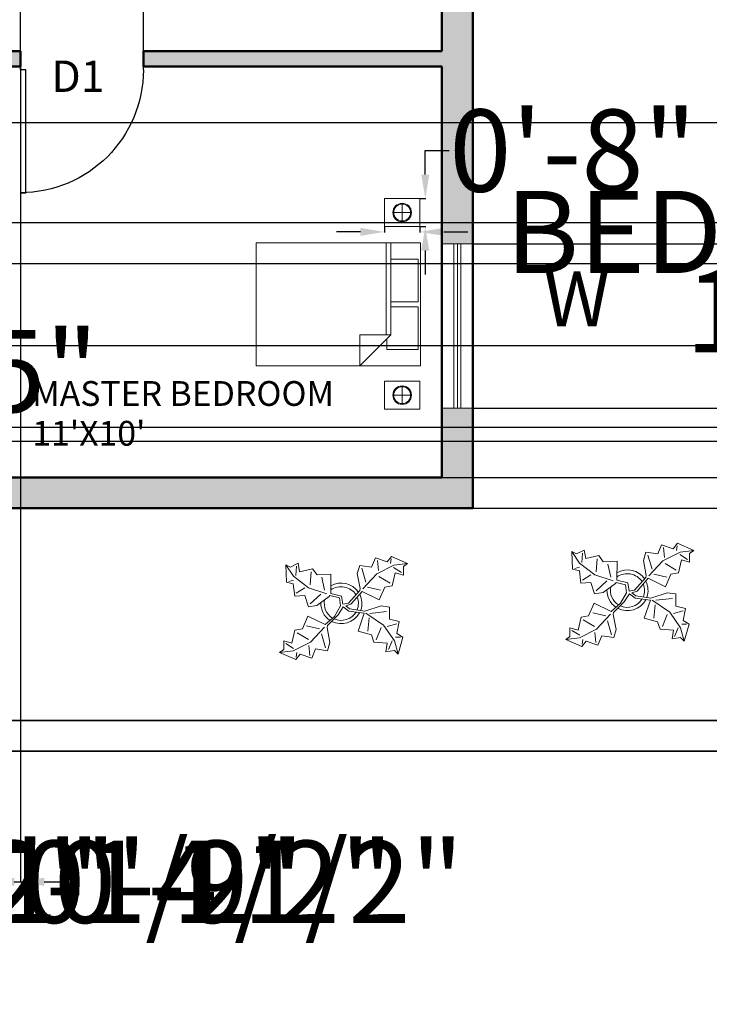
# Model space of a CAD drawing. Units: inches. Extents: x -166 to 1001, y 0 to 688.
# Tile 4 of 11: x 406 to 608, y 0 to 287. Entities that reach past the tile are written whole.
import ezdxf

# ---------------------------------------------------------------- set-up
doc = ezdxf.new("R2010")
doc.units = ezdxf.units.IN
doc.header["$MEASUREMENT"] = 0
for name, color, linetype, lineweight in [('A-ANNO-DIMS', 1, 'Continuous', 18), ('A-ANNO-TEXT', 2, 'Continuous', 25), ('A-AREA-IDEN', 2, 'Continuous', 25), ('A-DOOR', 6, 'Continuous', 25), ('A-GLAZ', 130, 'Continuous', 18), ('A-WALL-PATT', 5, 'Continuous', 13), ('C-SITE-WALL', 250, 'Continuous', 35), ('FURNITURE', 11, 'Continuous', 18), ('TREES', 80, 'Continuous', 13), ('WALLS', 250, 'Continuous', 50)]:
    doc.layers.add(name, color=color, linetype=linetype, lineweight=lineweight)
doc.styles.get("Standard").update_dxf_attribs({"font": 'arial.ttf'})
doc.dimstyles.get("Standard").update_dxf_attribs({"dimtxt": 24, "dimasz": 7, "dimexe": 0.18, "dimexo": 0.0625, "dimgap": 0.09, "dimtad": 0, "dimtih": 1, "dimtoh": 1, "dimdec": 0, "dimzin": 0, "dimdsep": 46, "dimlunit": 3, "dimtxsty": 'Standard', "dimcen": 0.09, "dimadec": 0, "dimazin": 0, "dimtfac": 1, "dimtdec": 0, "dimtofl": 0, "dimtmove": 0, "dimatfit": 3, "dimfxl": 1, "dimtolj": 1, "dimtzin": 0, "dimarcsym": 0})

# ---------------------------------------------------------------- blocks, each defined once
blk = doc.blocks.new('*U6')
for p, q in [((0, 0), (0, -6)), ((40, 0), (40, -6))]:
    blk.add_line(p, q)
blk.add_lwpolyline([(0, 0), (0, 40), (1.75, 40), (1.75, 0)], close=True)
blk.add_arc((0, 0), 40, 0, 90)
blk = doc.blocks.new('Bed - Queen')
for p, q in [((0, -80.00003), (0, 0)), ((0, 0), (59.99999, 0)), ((59.99999, 0), (59.99999, -80.00003)), ((7.99999, -1.2), (28.79998, -1.2)), ((7.99999, -14.4), (7.99999, -1.2)), ((28.79998, -1.2), (28.79998, -14.4)), ((31.19999, -1.2), (51.99999, -1.2)), ((31.19999, -14.4), (31.19999, -1.2)), ((51.99999, -1.2), (51.99999, -16.4)), ((0, -14.4), (44.8, -14.4)), ((44.8, -16.8), (0, -16.8)), ((59.99999, -29.6), (44.8, -14.4)), ((44.8, -14.4), (44.8, -29.6)), ((51.99999, -16.4), (46.79936, -16.4)), ((44.8, -29.6), (59.99999, -29.6)), ((59.99999, -80.00003), (0, -80.00003))]:
    blk.add_line(p, q)
blk = doc.blocks.new('Plant - Rubber or Philodendron')
for p, q in [((-14.8639, 10.7964), (-12.6195, 11.8975)), ((-12.6195, 11.8975), (-12.1909, 9.4345)), ((8.8871, 10.7908), (9.9809, 13.4933)), ((9.9809, 13.4933), (13.3837, 12.301)), ((10.5828, 12.6946), (10.8893, 9.7953)), ((13.3837, 12.301), (14.68, 13.9039)), ((14.5816, 13.2037), (14.3848, 11.8033)), ((14.68, 13.9039), (19.3848, 11.8146)), ((19.3848, 11.8146), (15.3859, 11.3055)), ((19.3848, 11.8146), (18.1868, 10.9119)), ((-16.2005, 11.4774), (-13.9899, 8.1064)), ((-16.2005, 11.4774), (-14.8639, 10.7964)), ((-16.0159, 6.3329), (-16.2005, 11.4774)), ((-13.3174, 8.325), (-13.0735, 11.0065)), ((-12.1909, 9.4345), (-8.3829, 10.3)), ((-8.8369, 9.409), (-9.0894, 5.6095)), ((-8.3829, 10.3), (-7.0549, 8.501)), ((-7.0549, 8.501), (-3.0284, 8.6941)), ((-3.0284, 8.6941), (-3.0709, 3.1041)), ((4.6914, 8.8812), (5.3859, 11.2828)), ((4.6914, 8.8812), (5.5014, 4.4831)), ((5.3859, 11.2828), (8.8871, 10.7908)), ((5.9878, 10.4842), (7.1971, 6.3869)), ((10.3916, 8.7942), (6.2847, 4.4028)), ((15.3859, 11.3055), (10.3916, 8.7942)), ((15.7909, 9.1065), (14.8995, 5.3044)), ((15.2875, 10.6053), (17.5907, 9.2105)), ((18.1925, 8.4119), (15.7909, 9.1065)), ((18.1868, 10.9119), (18.1925, 8.4119)), ((-14.0069, 5.8704), (-16.0159, 6.3329)), ((-15.3434, 6.5514), (-13.9984, 6.9884)), ((-13.5868, 2.2894), (-14.0069, 5.8704)), ((-13.9899, 8.1064), (-9.5434, 4.7185)), ((-4.8529, 4.012), (-5.7184, 7.82)), ((14.2977, 6.1031), (10.9934, 7.9956)), ((-13.1329, 3.1804), (-10.6614, 4.727)), ((-9.5434, 4.7185), (-4.1917, 2.9888)), ((-9.1318, 0.0195), (-5.9793, 2.9025)), ((-3.0709, 3.1041), (0.0797, 2.3163)), ((2.1141, 0.2298), (5.4346, 3.9146)), ((6.1032, 3.6844), (2.8262, -0.031)), ((5.4346, 3.9146), (5.5014, 4.4831)), ((11.1089, 1.1958), (6.1032, 3.6844)), ((7.7005, 4.8881), (11.5025, 3.9967)), ((12.7005, 4.8994), (11.1089, 1.1958)), ((14.8995, 5.3044), (12.7005, 4.8994)), ((-10.6784, 2.491), (-13.5868, 2.2894)), ((-9.5858, -0.8715), (-10.6784, 2.491)), ((-7.1228, -0.443), (-3.5248, 2.2131)), ((-3.5248, 2.2131), (-3.3011, 2.4355)), ((-3.3011, 2.4355), (-0.5306, 1.7947)), ((-0.5306, 1.7947), (-0.2255, -0.5527)), ((-0.5306, 1.7947), (-0.5306, 1.7947)), ((0.0797, 2.3163), (0.4866, -0.031)), ((0.4866, -0.031), (2.1141, 0.2298)), ((-7.1228, -0.443), (-9.5858, -0.8715)), ((-2.019, -3.6148), (-0.2255, -0.5527)), ((-0.9375, -3.1608), (0.5883, -0.8135)), ((0.5883, -0.8135), (2.2447, -2.0916)), ((2.8262, -0.031), (1.3003, -0.5527)), ((1.3003, -0.5527), (2.4193, -1.4655)), ((2.2447, -2.0916), (6.7108, -2.6626)), ((2.4193, -1.4655), (6.895, -2.1175)), ((4.943, -7.9659), (6.7108, -2.6626)), ((11.6605, -0.5413), (6.895, -2.1175)), ((12.3677, -6.1981), (7.219, -2.6772)), ((8.3544, -2.7453), (13.1973, -2.1704)), ((11.6605, -0.5413), (14.1354, -0.8948)), ((14.1354, -0.8948), (14.1354, -4.4304)), ((-11.3237, -7.2629), (-9.7321, -3.5593)), ((-9.7321, -3.5593), (-4.7264, -6.0479)), ((-2.019, -3.6148), (-4.7264, -6.0479)), ((-4.0579, -6.2781), (-0.9375, -3.1608)), ((8.125, -4.0768), (7.7715, -7.9659)), ((14.1354, -4.4304), (16.9638, -5.1375)), ((16.9638, -5.1375), (16.2567, -8.673)), ((-14.4141, -11.4699), (-13.5228, -7.6679)), ((-13.5228, -7.6679), (-11.3237, -7.2629)), ((-12.921, -8.4665), (-9.6166, -10.359)), ((-6.3237, -7.2516), (-10.1257, -6.3602)), ((-9.0148, -11.1577), (-4.9047, -6.8122)), ((-4.1246, -6.8466), (-4.0579, -6.2781)), ((-3.3146, -11.2447), (-4.1246, -6.8466)), ((8.8321, -9.0266), (4.943, -7.9659)), ((10.2463, -10.4408), (11.6605, -6.9053)), ((15.5496, -10.7943), (12.3677, -6.1981)), ((16.2567, -5.8446), (13.4283, -6.5517)), ((-16.8157, -10.7754), (-14.4141, -11.4699)), ((-16.8101, -13.2754), (-16.8157, -10.7754)), ((-14.0091, -13.669), (-9.0148, -11.1577)), ((-4.611, -12.8477), (-5.8203, -8.7504)), ((-3.3146, -11.2447), (-4.0092, -13.6463)), ((9.5392, -11.1479), (8.8321, -9.0266)), ((13.4283, -11.5015), (9.5392, -11.1479)), ((13.0748, -13.9763), (13.4283, -11.5015)), ((14.8425, -10.7943), (13.7819, -13.2692)), ((16.6103, -14.6834), (15.5496, -10.7943)), ((17.3174, -9.7337), (15.9032, -9.7337)), ((16.2567, -8.673), (18.0245, -9.7337)), ((18.0245, -9.7337), (16.6103, -14.6834)), ((-18.008, -14.1781), (-16.8101, -13.2754)), ((-18.008, -14.1781), (-14.0091, -13.669)), ((-13.3032, -16.2674), (-18.008, -14.1781)), ((-13.9107, -12.9688), (-16.2139, -11.574)), ((-13.2048, -15.5672), (-13.008, -14.1668)), ((-9.206, -15.0581), (-9.5126, -12.1588)), ((-7.5103, -13.1543), (-8.6042, -15.8568)), ((-4.0092, -13.6463), (-7.5103, -13.1543)), ((15.5496, -13.6228), (13.0748, -13.9763)), ((16.6103, -14.6834), (15.5496, -13.6228)), ((-12.0069, -14.6645), (-13.3032, -16.2674)), ((-8.6042, -15.8568), (-12.0069, -14.6645))]:
    blk.add_line(p, q)
for centre, radius, start, end in [((0, 0), 6.1275, 34.37569, 120.1028), ((-0.0601, -0.2075), 5.2461, 33.82192, 124.9414), ((0.0308, 0.1664), 6, 178.6147, 235.1169), ((0.0308, 0.1664), 5, 168.1647, 238.6725), ((-0.2664, 0.1682), 5.2775, 338.4094, 20.03007), ((-0.098, 0.1364), 6.1288, 341.2017, 26.09184), ((-0.0234, 0.3825), 6.1492, 242.5812, 331.2714), ((-0.1102, 0.4886), 5.2883, 247.3711, 327.472)]:
    blk.add_arc(centre, radius, start, end)
blk = doc.blocks.new('WIN-48IN')
for p, q in [((0, 4.5), (0, 9)), ((0, 9), (0, 0)), ((48, 9), (48, 0)), ((0, 5.5), (48, 5.5)), ((0, 4.5), (48, 4.5)), ((0, 3.5), (48, 3.5))]:
    blk.add_line(p, q)
blk = doc.blocks.new('BEDSIDE-TABLE-LAMP')
for p, q in [((5.2, 1.64), (5.2, 6.55)), ((2.75, 4.1), (7.66, 4.1))]:
    blk.add_line(p, q)
blk.add_lwpolyline([(0, 8.19), (10.4, 8.19), (10.4, 0), (0, 0)], close=True)
for radius in [2.71, 2.71, 2.71, 2.46]:
    blk.add_circle((5.2, 4.1), radius)
blk = doc.blocks.new('*D21')
at = {"layer": 'A-ANNO-DIMS', "color": 0, "lineweight": -2, "transparency": 16777216}
for p, q in [((506.04, 225.45), (499.04, 225.45)), ((513.04, 226.95), (513.04, 225.27)), ((523.44, 226.95), (523.44, 225.27)), ((530.44, 225.45), (537.44, 225.45))]:
    blk.add_line(p, q, dxfattribs=at)
at = {"layer": 'A-ANNO-DIMS', "color": 0, "transparency": 16777216}
for points in [[(506.04, 226.62), (506.04, 224.29), (513.04, 225.45)], [(530.44, 226.62), (530.44, 224.29), (523.44, 225.45)]]:
    blk.add_solid(points, dxfattribs=at)
at = {"layer": 'Defpoints', "color": 0, "transparency": 16777216}
for p in [(513.04, 227.01), (523.44, 227.01), (523.44, 225.45)]:
    blk.add_point(p, dxfattribs=at)
at = {"layer": 'A-ANNO-DIMS', "color": 0, "transparency": 16777216, "insert": (775.99, 225.45), "char_height": 24, "attachment_point": 5}
blk.add_mtext('\\A1;BEDSIDE LAMP 0\'-10 1/2" TYP.', dxfattribs=at)
blk = doc.blocks.new('*D22')
at = {"layer": 'A-ANNO-DIMS', "color": 0, "lineweight": -2, "transparency": 16777216}
for p, q in [((525, 242.21), (525, 249.21)), ((525, 249.21), (532, 249.21)), ((523.5, 235.21), (525.18, 235.21)), ((523.5, 227.01), (525.18, 227.01)), ((525, 220.01), (525, 213.01))]:
    blk.add_line(p, q, dxfattribs=at)
at = {"layer": 'A-ANNO-DIMS', "color": 0, "transparency": 16777216}
for points in [[(523.83, 242.21), (526.17, 242.21), (525, 235.21)], [(523.83, 220.01), (526.17, 220.01), (525, 227.01)]]:
    blk.add_solid(points, dxfattribs=at)
at = {"layer": 'Defpoints', "color": 0, "transparency": 16777216}
for p in [(523.44, 235.21), (525, 235.21), (523.44, 227.01)]:
    blk.add_point(p, dxfattribs=at)
at = {"layer": 'A-ANNO-DIMS', "color": 0, "transparency": 16777216, "insert": (605.24, 249.21), "char_height": 24, "attachment_point": 5}
blk.add_mtext('\\A1;0\'-8" TYP.', dxfattribs=at)
blk = doc.blocks.new('*D28')
at = {"layer": 'A-ANNO-DIMS', "color": 0, "lineweight": -2, "transparency": 16777216}
for p, q in [((355.46, 177.8), (355.46, 184.8)), ((355.46, 184.8), (362.46, 184.8)), ((351.57, 177.8), (355.64, 177.8)), ((355.46, 168.04), (355.46, 170.8)), ((351.57, 161.04), (355.64, 161.04))]:
    blk.add_line(p, q, dxfattribs=at)
at = {"layer": 'A-ANNO-DIMS', "color": 0, "transparency": 16777216}
for points in [[(354.29, 170.8), (356.63, 170.8), (355.46, 177.8)], [(354.29, 168.04), (356.63, 168.04), (355.46, 161.04)]]:
    blk.add_solid(points, dxfattribs=at)
at = {"layer": 'Defpoints', "color": 0, "transparency": 16777216}
for p in [(351.51, 177.8), (355.46, 177.8), (351.51, 161.04)]:
    blk.add_point(p, dxfattribs=at)
at = {"layer": 'A-ANNO-DIMS', "color": 0, "transparency": 16777216, "insert": (393.32, 184.8), "char_height": 24, "attachment_point": 5}
blk.add_mtext('\\A1;1\'-5"', dxfattribs=at)
blk = doc.blocks.new('*D46')
at = {"layer": 'A-ANNO-DIMS', "color": 0, "lineweight": -2, "transparency": 16777216}
for p, q in [((261.38, 474.68), (261.38, 35.41)), ((298.66, 474.68), (298.66, 35.41)), ((268.38, 35.59), (291.66, 35.59)), ((298.66, 35.59), (305.66, 35.59))]:
    blk.add_line(p, q, dxfattribs=at)
at = {"layer": 'A-ANNO-DIMS', "color": 0, "transparency": 16777216}
for points in [[(268.38, 36.76), (268.38, 34.42), (261.38, 35.59)], [(291.66, 36.76), (291.66, 34.42), (298.66, 35.59)]]:
    blk.add_solid(points, dxfattribs=at)
at = {"layer": 'Defpoints', "color": 0, "transparency": 16777216}
for p in [(261.38, 474.74), (298.66, 474.74), (298.66, 35.59)]:
    blk.add_point(p, dxfattribs=at)
at = {"layer": 'A-ANNO-DIMS', "color": 0, "transparency": 16777216, "insert": (365.61, 35.59), "char_height": 24, "attachment_point": 5}
blk.add_mtext('\\A1;3\'-1 1/2"', dxfattribs=at)
blk = doc.blocks.new('*D50')
at = {"layer": 'A-ANNO-DIMS', "color": 0, "lineweight": -2, "transparency": 16777216}
for p, q in [((284.58, 144.68), (284.58, 35.41)), ((358.23, 144.68), (358.23, 35.41)), ((291.58, 35.59), (351.23, 35.59)), ((358.23, 35.59), (365.23, 35.59))]:
    blk.add_line(p, q, dxfattribs=at)
at = {"layer": 'A-ANNO-DIMS', "color": 0, "transparency": 16777216}
for points in [[(291.58, 36.76), (291.58, 34.42), (284.58, 35.59)], [(351.23, 36.76), (351.23, 34.42), (358.23, 35.59)]]:
    blk.add_solid(points, dxfattribs=at)
at = {"layer": 'Defpoints', "color": 0, "transparency": 16777216}
for p in [(284.58, 144.74), (358.23, 144.74), (358.23, 35.59)]:
    blk.add_point(p, dxfattribs=at)
at = {"layer": 'A-ANNO-DIMS', "color": 0, "transparency": 16777216, "insert": (425.24, 35.59), "char_height": 24, "attachment_point": 5}
blk.add_mtext('\\A1;6\'-1 1/2"', dxfattribs=at)
blk = doc.blocks.new('*D51')
at = {"layer": 'A-ANNO-DIMS', "color": 0, "lineweight": -2, "transparency": 16777216}
for p, q in [((675.03, 168.41), (675.03, 175.41)), ((675.03, 175.41), (682.03, 175.41)), ((24.44, 168.41), (675.21, 168.41)), ((675.03, 160.74), (675.03, 161.41)), ((24.44, 153.74), (675.21, 153.74))]:
    blk.add_line(p, q, dxfattribs=at)
at = {"layer": 'A-ANNO-DIMS', "color": 0, "transparency": 16777216}
for points in [[(673.87, 161.41), (676.2, 161.41), (675.03, 168.41)], [(673.87, 160.74), (676.2, 160.74), (675.03, 153.74)]]:
    blk.add_solid(points, dxfattribs=at)
at = {"layer": 'Defpoints', "color": 0, "transparency": 16777216}
for p in [(24.38, 168.41), (675.03, 168.41), (24.38, 153.74)]:
    blk.add_point(p, dxfattribs=at)
at = {"layer": 'A-ANNO-DIMS', "color": 0, "transparency": 16777216, "insert": (740.85, 175.41), "char_height": 24, "attachment_point": 5}
blk.add_mtext('\\A1;1\'-2 1/2"', dxfattribs=at)
blk = doc.blocks.new('*D53')
at = {"layer": 'A-ANNO-DIMS', "color": 0, "lineweight": -2, "transparency": 16777216}
for p, q in [((675.03, 180.94), (675.03, 187.94)), ((538.94, 173.94), (675.21, 173.94)), ((538.94, 144.74), (675.21, 144.74)), ((675.03, 137.74), (675.03, 130.74))]:
    blk.add_line(p, q, dxfattribs=at)
at = {"layer": 'A-ANNO-DIMS', "color": 0, "transparency": 16777216}
for points in [[(673.87, 180.94), (676.2, 180.94), (675.03, 173.94)], [(673.87, 137.74), (676.2, 137.74), (675.03, 144.74)]]:
    blk.add_solid(points, dxfattribs=at)
at = {"layer": 'Defpoints', "color": 0, "transparency": 16777216}
for p in [(538.88, 173.94), (675.03, 173.94), (538.88, 144.74)]:
    blk.add_point(p, dxfattribs=at)
at = {"layer": 'A-ANNO-DIMS', "color": 0, "transparency": 16777216, "insert": (675.03, 159.34), "char_height": 24, "attachment_point": 5}
blk.add_mtext('\\A1;2\'-5"', dxfattribs=at)
blk = doc.blocks.new('*D54')
at = {"layer": 'A-ANNO-DIMS', "color": 0, "lineweight": -2, "transparency": 16777216}
for p, q in [((538.94, 298.79), (675.21, 298.79)), ((675.03, 291.79), (675.03, 272.71)), ((675.03, 228.94), (675.03, 248.02)), ((538.94, 221.94), (675.21, 221.94))]:
    blk.add_line(p, q, dxfattribs=at)
at = {"layer": 'A-ANNO-DIMS', "color": 0, "transparency": 16777216}
for points in [[(673.87, 291.79), (676.2, 291.79), (675.03, 298.79)], [(673.87, 228.94), (676.2, 228.94), (675.03, 221.94)]]:
    blk.add_solid(points, dxfattribs=at)
at = {"layer": 'Defpoints', "color": 0, "transparency": 16777216}
for p in [(538.88, 298.79), (675.03, 298.79), (538.88, 221.94)]:
    blk.add_point(p, dxfattribs=at)
at = {"layer": 'A-ANNO-DIMS', "color": 0, "transparency": 16777216, "insert": (675.03, 260.36), "char_height": 24, "attachment_point": 5}
blk.add_mtext('\\A1;6\'-5"', dxfattribs=at)
blk = doc.blocks.new('*D55')
at = {"layer": 'A-ANNO-DIMS', "color": 0, "lineweight": -2, "transparency": 16777216}
for p, q in [((-120.77, 341.73), (-120.77, 348.73)), ((529.82, 334.73), (-120.95, 334.73)), ((529.82, 298.79), (-120.95, 298.79)), ((-120.77, 291.79), (-120.77, 284.79))]:
    blk.add_line(p, q, dxfattribs=at)
at = {"layer": 'A-ANNO-DIMS', "color": 0, "transparency": 16777216}
for points in [[(-121.93, 341.73), (-119.6, 341.73), (-120.77, 334.73)], [(-121.93, 291.79), (-119.6, 291.79), (-120.77, 298.79)]]:
    blk.add_solid(points, dxfattribs=at)
at = {"layer": 'Defpoints', "color": 0, "transparency": 16777216}
for p in [(-120.77, 334.73), (529.88, 334.73), (529.88, 298.79)]:
    blk.add_point(p, dxfattribs=at)
at = {"layer": 'A-ANNO-DIMS', "color": 0, "transparency": 16777216, "insert": (-120.77, 316.76), "char_height": 24, "attachment_point": 5}
blk.add_mtext('\\A1;3\'-0"', dxfattribs=at)
blk = doc.blocks.new('*D63')
at = {"layer": 'A-ANNO-DIMS', "color": 0, "lineweight": -2, "transparency": 16777216}
for p, q in [((274.49, 338.18), (274.49, 35.41)), ((384.24, 338.18), (384.24, 35.41)), ((281.49, 35.59), (377.24, 35.59)), ((384.24, 35.59), (391.24, 35.59))]:
    blk.add_line(p, q, dxfattribs=at)
at = {"layer": 'A-ANNO-DIMS', "color": 0, "transparency": 16777216}
for points in [[(281.49, 36.76), (281.49, 34.42), (274.49, 35.59)], [(377.24, 36.76), (377.24, 34.42), (384.24, 35.59)]]:
    blk.add_solid(points, dxfattribs=at)
at = {"layer": 'Defpoints', "color": 0, "transparency": 16777216}
for p in [(274.49, 338.24), (384.24, 338.24), (384.24, 35.59)]:
    blk.add_point(p, dxfattribs=at)
at = {"layer": 'A-ANNO-DIMS', "color": 0, "transparency": 16777216, "insert": (451.19, 35.59), "char_height": 24, "attachment_point": 5}
blk.add_mtext('\\A1;9\'-1 1/2"', dxfattribs=at)
blk = doc.blocks.new('*D71')
at = {"layer": 'A-ANNO-DIMS', "color": 0, "lineweight": -2, "transparency": 16777216}
for p, q in [((406.66, 278.3), (406.66, 593.07)), ((413.66, 592.89), (435.61, 592.89)), ((442.61, 278.3), (442.61, 593.07)), ((442.61, 592.89), (449.61, 592.89))]:
    blk.add_line(p, q, dxfattribs=at)
at = {"layer": 'A-ANNO-DIMS', "color": 0, "transparency": 16777216}
for points in [[(413.66, 594.06), (413.66, 591.72), (406.66, 592.89)], [(435.61, 594.06), (435.61, 591.72), (442.61, 592.89)]]:
    blk.add_solid(points, dxfattribs=at)
at = {"layer": 'Defpoints', "color": 0, "transparency": 16777216}
for p in [(442.61, 592.89), (406.66, 278.24), (442.61, 278.24)]:
    blk.add_point(p, dxfattribs=at)
at = {"layer": 'A-ANNO-DIMS', "color": 0, "transparency": 16777216, "insert": (481.59, 592.89), "char_height": 24, "attachment_point": 5}
blk.add_mtext('\\A1;3\'-0"', dxfattribs=at)
blk = doc.blocks.new('*D72')
at = {"layer": 'A-ANNO-DIMS', "color": 0, "lineweight": -2, "transparency": 16777216}
for p, q in [((397.88, 273.68), (397.88, 35.41)), ((406.66, 273.68), (406.66, 35.41)), ((390.88, 35.59), (383.88, 35.59)), ((413.66, 35.59), (420.66, 35.59))]:
    blk.add_line(p, q, dxfattribs=at)
at = {"layer": 'A-ANNO-DIMS', "color": 0, "transparency": 16777216}
for points in [[(390.88, 36.76), (390.88, 34.42), (397.88, 35.59)], [(413.66, 36.76), (413.66, 34.42), (406.66, 35.59)]]:
    blk.add_solid(points, dxfattribs=at)
at = {"layer": 'Defpoints', "color": 0, "transparency": 16777216}
for p in [(397.88, 273.74), (406.66, 273.74), (406.66, 35.59)]:
    blk.add_point(p, dxfattribs=at)
at = {"layer": 'A-ANNO-DIMS', "color": 0, "transparency": 16777216, "insert": (452.65, 35.59), "char_height": 24, "attachment_point": 5}
blk.add_mtext('\\A1;0\'-9"', dxfattribs=at)
blk = doc.blocks.new('*D74')
at = {"layer": 'A-ANNO-DIMS', "color": 0, "lineweight": -2, "transparency": 16777216}
for p, q in [((675.03, 171.32), (675.03, 178.32)), ((675.03, 178.32), (682.03, 178.32)), ((397.94, 164.32), (675.21, 164.32)), ((397.94, 153.74), (675.21, 153.74)), ((675.03, 146.74), (675.03, 139.74))]:
    blk.add_line(p, q, dxfattribs=at)
at = {"layer": 'A-ANNO-DIMS', "color": 0, "transparency": 16777216}
for points in [[(673.87, 171.32), (676.2, 171.32), (675.03, 164.32)], [(673.87, 146.74), (676.2, 146.74), (675.03, 153.74)]]:
    blk.add_solid(points, dxfattribs=at)
at = {"layer": 'Defpoints', "color": 0, "transparency": 16777216}
for p in [(397.88, 164.32), (675.03, 164.32), (397.88, 153.74)]:
    blk.add_point(p, dxfattribs=at)
at = {"layer": 'A-ANNO-DIMS', "color": 0, "transparency": 16777216, "insert": (751.31, 178.32), "char_height": 24, "attachment_point": 5}
blk.add_mtext('\\A1;0\'-10 1/2"', dxfattribs=at)
blk = doc.blocks.new('*D76')
at = {"layer": 'A-ANNO-DIMS', "color": 0, "lineweight": -2, "transparency": 16777216}
for p, q in [((675.03, 235.24), (675.03, 242.24)), ((160.94, 228.24), (675.21, 228.24)), ((160.94, 216.24), (675.21, 216.24)), ((675.03, 209.24), (675.03, 202.24)), ((675.03, 202.24), (668.03, 202.24))]:
    blk.add_line(p, q, dxfattribs=at)
at = {"layer": 'A-ANNO-DIMS', "color": 0, "transparency": 16777216}
for points in [[(673.87, 235.24), (676.2, 235.24), (675.03, 228.24)], [(673.87, 209.24), (676.2, 209.24), (675.03, 216.24)]]:
    blk.add_solid(points, dxfattribs=at)
at = {"layer": 'Defpoints', "color": 0, "transparency": 16777216}
for p in [(160.88, 228.24), (160.88, 216.24), (675.03, 216.24)]:
    blk.add_point(p, dxfattribs=at)
at = {"layer": 'A-ANNO-DIMS', "color": 0, "transparency": 16777216, "insert": (637.17, 202.24), "char_height": 24, "attachment_point": 5}
blk.add_mtext('\\A1;1\'-0"', dxfattribs=at)
blk = doc.blocks.new('*D77')
at = {"layer": 'A-ANNO-DIMS', "color": 0, "lineweight": -2, "transparency": 16777216}
for p, q in [((675.03, 199.24), (675.03, 206.24)), ((292.83, 192.24), (675.21, 192.24)), ((292.83, 153.74), (675.21, 153.74)), ((675.03, 146.74), (675.03, 139.74))]:
    blk.add_line(p, q, dxfattribs=at)
at = {"layer": 'A-ANNO-DIMS', "color": 0, "transparency": 16777216}
for points in [[(673.87, 199.24), (676.2, 199.24), (675.03, 192.24)], [(673.87, 146.74), (676.2, 146.74), (675.03, 153.74)]]:
    blk.add_solid(points, dxfattribs=at)
at = {"layer": 'Defpoints', "color": 0, "transparency": 16777216}
for p in [(292.77, 192.24), (292.77, 153.74), (675.03, 153.74)]:
    blk.add_point(p, dxfattribs=at)
at = {"layer": 'A-ANNO-DIMS', "color": 0, "transparency": 16777216, "insert": (675.03, 172.99), "char_height": 24, "attachment_point": 5}
blk.add_mtext('\\A1;3\'-2 1/2"', dxfattribs=at)
blk = doc.blocks.new('*D79')
at = {"layer": 'A-ANNO-DIMS', "color": 0, "lineweight": -2, "transparency": 16777216}
for p, q in [((208.68, 257.42), (675.21, 257.42)), ((675.03, 250.42), (675.03, 218.08)), ((675.03, 160.74), (675.03, 193.08)), ((292.83, 153.74), (675.21, 153.74))]:
    blk.add_line(p, q, dxfattribs=at)
at = {"layer": 'A-ANNO-DIMS', "color": 0, "transparency": 16777216}
for points in [[(673.87, 250.42), (676.2, 250.42), (675.03, 257.42)], [(673.87, 160.74), (676.2, 160.74), (675.03, 153.74)]]:
    blk.add_solid(points, dxfattribs=at)
at = {"layer": 'Defpoints', "color": 0, "transparency": 16777216}
for p in [(208.62, 257.42), (292.77, 153.74), (675.03, 153.74)]:
    blk.add_point(p, dxfattribs=at)
at = {"layer": 'A-ANNO-DIMS', "color": 0, "transparency": 16777216, "insert": (675.03, 205.58), "char_height": 24, "attachment_point": 5}
blk.add_mtext('\\A1;8\'-7 1/2"', dxfattribs=at)
blk = doc.blocks.new('*D80')
at = {"layer": 'A-ANNO-DIMS', "color": 0, "lineweight": -2, "transparency": 16777216}
for p, q in [((393.38, 383.15), (393.38, 35.41)), ((397.88, 383.15), (397.88, 35.41)), ((386.38, 35.59), (379.38, 35.59)), ((404.88, 35.59), (411.88, 35.59))]:
    blk.add_line(p, q, dxfattribs=at)
at = {"layer": 'A-ANNO-DIMS', "color": 0, "transparency": 16777216}
for points in [[(386.38, 36.76), (386.38, 34.42), (393.38, 35.59)], [(404.88, 36.76), (404.88, 34.42), (397.88, 35.59)]]:
    blk.add_solid(points, dxfattribs=at)
at = {"layer": 'Defpoints', "color": 0, "transparency": 16777216}
for p in [(393.38, 383.21), (397.88, 383.21), (397.88, 35.59)]:
    blk.add_point(p, dxfattribs=at)
at = {"layer": 'A-ANNO-DIMS', "color": 0, "transparency": 16777216, "insert": (471.83, 35.59), "char_height": 24, "attachment_point": 5}
blk.add_mtext('\\A1;0\'-4 1/2"', dxfattribs=at)

msp = doc.modelspace()

# ---------------------------------------------------------------- hatches: boundary and pattern name
at = {"layer": 'A-WALL-PATT'}
h = msp.add_hatch(color=256, dxfattribs=at)
h.dxf.hatch_style = 1
h.paths.add_polyline_path([(96.05, 483.74), (15.38, 483.74), (15.38, 414.29), (24.38, 414.29), (24.38, 474.74), (96.05, 474.74)])
h.paths.add_polyline_path([(175.47, 483.74), (144.05, 483.74), (144.05, 474.74), (156.38, 474.74), (175.47, 474.74)])
h.paths.add_polyline_path([(298.66, 483.74), (199.47, 483.74), (199.47, 474.74), (256.88, 474.74), (298.66, 474.74)])
h.paths.add_polyline_path([(430.46, 483.74), (346.66, 483.74), (346.66, 474.74), (393.38, 474.74), (430.46, 474.74)])
h.paths.add_polyline_path([(261.38, 474.74), (256.88, 474.74), (256.88, 342.74), (201.55, 342.74), (201.55, 338.24), (274.49, 338.24), (274.49, 342.74), (261.38, 342.74)])
h.paths.add_polyline_path([(160.88, 474.74), (156.38, 474.74), (156.38, 342.74), (146.03, 342.74), (146.03, 338.24), (171.55, 338.24), (171.55, 342.74), (160.88, 342.74)])
h.paths.add_polyline_path([(397.88, 474.74), (393.38, 474.74), (393.38, 383.21), (397.88, 383.21)])
h.paths.add_polyline_path([(538.88, 362.18), (529.88, 362.18), (529.88, 342.74), (397.88, 342.74), (397.88, 348.69), (393.38, 348.69), (393.38, 342.74), (384.24, 342.74), (384.24, 338.24), (529.88, 338.24), (529.88, 334.73), (538.88, 334.73)])
h.paths.add_polyline_path([(538.88, 483.74), (478.46, 483.74), (478.46, 474.74), (529.88, 474.74), (529.88, 410.18), (538.88, 410.18)])
h.paths.add_polyline_path([(538.88, 298.79), (529.88, 298.79), (529.88, 278.24), (442.61, 278.24), (442.61, 273.74), (529.88, 273.74), (529.88, 221.94), (538.88, 221.94)])
h.paths.add_polyline_path([(538.88, 173.94), (529.88, 173.94), (529.88, 153.74), (393.38, 153.74), (382.23, 153.74), (382.23, 144.74), (538.88, 144.74)])
h.paths.add_polyline_path([(397.88, 164.32), (393.38, 164.32), (393.38, 153.74), (397.88, 153.74)], flags=17)
h.paths.add_polyline_path([(397.88, 273.74), (406.66, 273.74), (406.66, 278.24), (393.38, 278.24), (393.38, 273.74), (393.38, 230.24), (316.88, 230.24), (316.88, 153.74), (321.38, 153.74), (321.38, 225.74), (393.38, 225.74), (393.38, 194.32), (397.88, 194.32)])
h.paths.add_polyline_path([(358.23, 153.74), (316.88, 153.74), (284.58, 153.74), (284.58, 144.74), (358.23, 144.74)])
h.paths.add_polyline_path([(224.58, 153.74), (156.38, 153.74), (149.31, 153.74), (149.31, 144.74), (224.58, 144.74)])
h.paths.add_polyline_path([(101.31, 153.74), (24.38, 153.74), (24.38, 168.41), (15.38, 168.41), (15.38, 144.74), (101.31, 144.74)])
h.paths.add_polyline_path([(160.88, 273.74), (160.88, 278.24), (147.87, 278.24), (147.87, 273.74), (156.38, 273.74), (156.38, 153.74), (160.88, 153.74)])
h.paths.add_polyline_path([(111.92, 278.24), (100.88, 278.24), (100.88, 338.24), (110.03, 338.24), (110.03, 342.74), (24.38, 342.74), (24.38, 366.29), (15.38, 366.29), (15.38, 216.41), (24.38, 216.41), (24.38, 273.74), (44.93, 273.74), (44.93, 278.24), (24.38, 278.24), (24.38, 338.24), (96.38, 338.24), (96.38, 278.24), (74.93, 278.24), (74.93, 273.74), (111.92, 273.74)])

# ---------------------------------------------------------------- linework, layer by layer
at = {"layer": 'C-SITE-WALL'}
for p, q in [((-73.62, 82.74), (627.88, 82.74)), ((-82.62, 73.74), (636.88, 73.74))]:
    msp.add_line(p, q, dxfattribs=at)
at = {"layer": 'WALLS'}
for p, q in [((538.88, 144.74), (538.88, 483.74)), ((529.88, 278.24), (529.88, 298.97)), ((393.38, 278.24), (406.66, 278.24)), ((406.66, 278.24), (406.66, 273.74)), ((442.61, 278.24), (529.88, 278.24)), ((442.61, 273.74), (442.61, 278.24)), ((397.88, 273.74), (406.66, 273.74)), ((442.61, 273.74), (529.88, 273.74)), ((529.88, 153.74), (529.88, 273.74)), ((393.38, 153.74), (529.88, 153.74)), ((15.38, 144.74), (538.88, 144.74))]:
    msp.add_line(p, q, dxfattribs=at)

# ---------------------------------------------------------------- block references
at = {"layer": 'A-DOOR', "xscale": -0.8986699555462259, "yscale": 0.8986699555462259, "zscale": 0.8986699555462259, "rotation": 180}
msp.add_blockref('*U6', (406.66, 272.85), dxfattribs=at)
at = {"layer": 'A-GLAZ', "rotation": 89.99999999999923}
msp.add_blockref('WIN-48IN', (538.88, 173.94), dxfattribs=at)
at = {"layer": 'FURNITURE'}
for p in [(513.04, 227.01), (513.04, 173.67)]:
    msp.add_blockref('BEDSIDE-TABLE-LAMP', p, dxfattribs=at)
at = {"layer": 'FURNITURE', "xscale": 0.6000001000000168, "yscale": 0.6000001000000168, "zscale": 0.6000001000000168, "rotation": 270}
msp.add_blockref('Bed - Queen', (523.6, 222.3), dxfattribs=at)
at = {"layer": 'TREES'}
for p in [(584.07, 120.57), (500.44, 116.76)]:
    msp.add_blockref('Plant - Rubber or Philodendron', p, dxfattribs=at)

# ---------------------------------------------------------------- texts
at = {"layer": 'A-ANNO-TEXT'}
for s, height, p in [('D1', 9.17, (415.7, 266.34)), ('W ', 16.096, (559.64, 197.82))]:
    msp.add_text(s, height=height, dxfattribs=at).set_placement(p)
at = {"layer": 'A-AREA-IDEN'}
for s, height, p in [('MASTER BEDROOM', 7.2392, (410.14, 174.63)), ("11'X10'", 7.239, (410.14, 163))]:
    msp.add_text(s, height=height, dxfattribs=at).set_placement(p)

# ---------------------------------------------------------------- dimensions: what is measured, and where the dimension line sits
at = {"layer": 'A-ANNO-DIMS'}
for base, p1, p2, picture, middle in [((442.6082, 592.8909), (406.6614, 278.2409), (442.6082, 278.2409), '*D71', (481.589, 592.8909)), ((298.66, 35.59), (261.38, 474.74), (298.66, 474.74), '*D46', (365.61, 35.59)), ((397.88, 35.59), (393.38, 383.21), (397.88, 383.21), '*D80', (471.83, 35.59)), ((384.2404, 35.5909), (274.4932, 338.2409), (384.2404, 338.2409), '*D63', (451.1912, 35.5909)), ((406.66, 35.59), (397.88, 273.74), (406.66, 273.74), '*D72', (452.65, 35.59)), ((358.2261, 35.5909), (284.5839, 144.7409), (358.2261, 144.7409), '*D50', (425.2425, 35.5909))]:
    dim = msp.add_linear_dim(base=base, p1=p1, p2=p2, dimstyle='Standard', override={"dimdec": 1, "dimlfac": 1, "dimrnd": 0, "dimzin": 1, "dimdsep": 46, "dimlunit": 4, "dimfrac": 2}, dxfattribs=at)
    dim.commit()
    dim.dimension.update_dxf_attribs({"geometry": picture, "text_midpoint": middle})
for base, p1, p2, picture, middle in [((-120.77, 334.73), (529.88, 298.79), (529.88, 334.73), '*D55', (-120.77, 316.76)), ((675.0325, 298.7872), (538.8825, 221.9421), (538.8825, 298.7872), '*D54', (675.0325, 260.3646)), ((675.03, 153.74), (208.62, 257.42), (292.77, 153.74), '*D79', (675.03, 205.58)), ((675.03, 216.24), (160.88, 228.24), (160.88, 216.24), '*D76', (637.17, 202.24)), ((675.03, 164.32), (397.88, 153.74), (397.88, 164.32), '*D74', (751.31, 178.32)), ((675.03, 168.41), (24.38, 153.74), (24.38, 168.41), '*D51', (740.85, 175.41)), ((675.03, 153.74), (292.77, 192.24), (292.77, 153.74), '*D77', (675.03, 172.99)), ((355.46, 177.8), (351.51, 161.04), (351.51, 177.8), '*D28', (393.32, 184.8)), ((675.03, 173.94), (538.88, 144.74), (538.88, 173.94), '*D53', (675.03, 159.34))]:
    dim = msp.add_linear_dim(base=base, p1=p1, p2=p2, angle=90, dimstyle='Standard', override={"dimdec": 1, "dimlfac": 1, "dimrnd": 0, "dimzin": 1, "dimdsep": 46, "dimlunit": 4, "dimfrac": 2}, dxfattribs=at)
    dim.commit()
    dim.dimension.update_dxf_attribs({"geometry": picture, "text_midpoint": middle})
dim = msp.add_linear_dim(base=(523.44, 225.45), p1=(513.04, 227.01), p2=(523.44, 227.01), text='BEDSIDE LAMP <> TYP.', dimstyle='Standard', override={"dimdec": 1, "dimlfac": 1, "dimrnd": 0, "dimzin": 1, "dimdsep": 46, "dimlunit": 4, "dimfrac": 2}, dxfattribs=at)
dim.commit()
dim.dimension.update_dxf_attribs({"geometry": '*D21', "text_midpoint": (775.99, 225.45)})
dim = msp.add_linear_dim(base=(525, 235.21), p1=(523.44, 227.01), p2=(523.44, 235.21), angle=90, text='<> TYP.', dimstyle='Standard', override={"dimdec": 1, "dimlfac": 1, "dimrnd": 0, "dimzin": 1, "dimdsep": 46, "dimlunit": 4, "dimfrac": 2}, dxfattribs=at)
dim.commit()
dim.dimension.update_dxf_attribs({"geometry": '*D22', "text_midpoint": (605.24, 249.21)})

doc.saveas('drawing.dxf')
